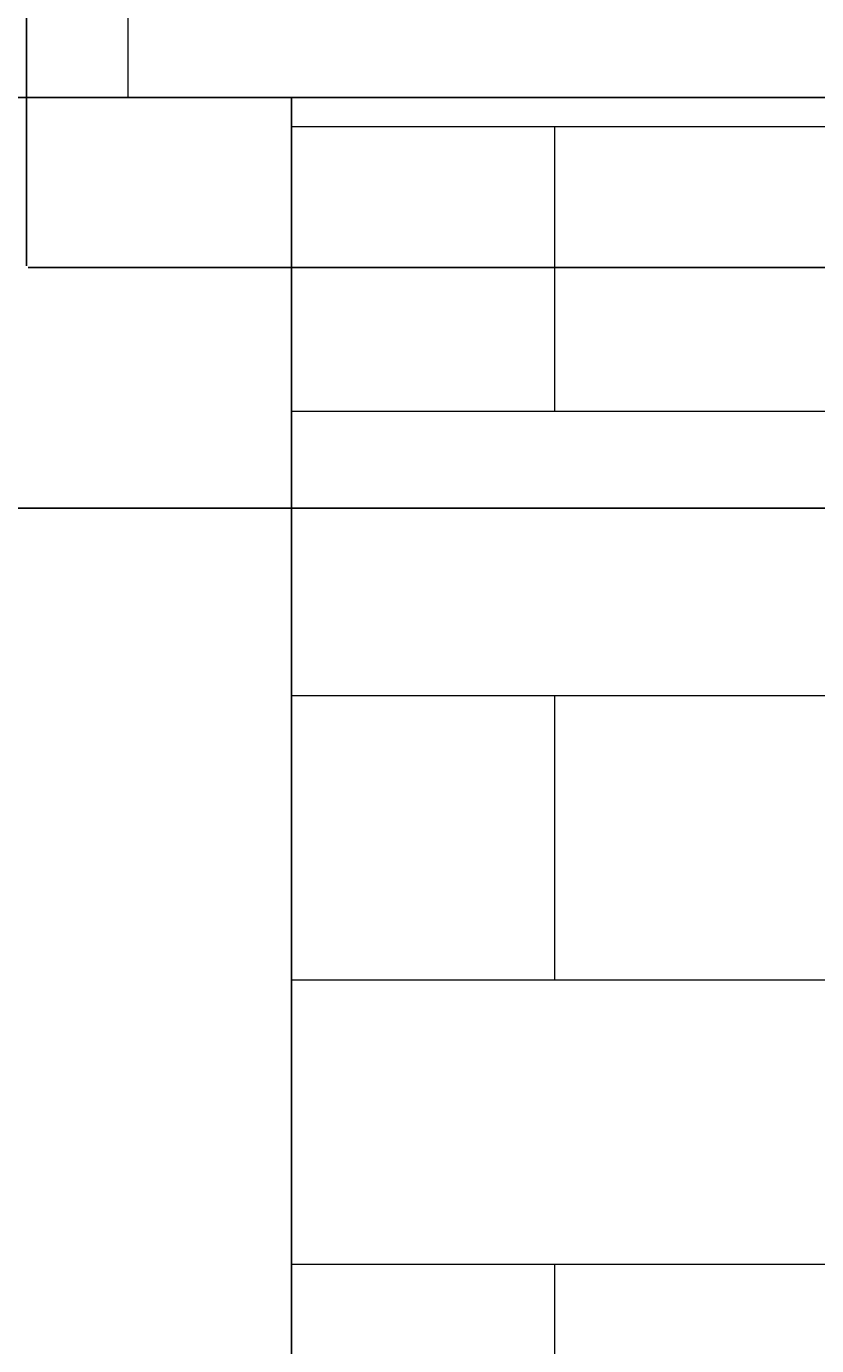
# Model space of a CAD drawing. Units: inches. Extents: x 37 to 824, y -700 to 234.
# Tile 18 of 77: x 348 to 378, y -536 to -487. Entities that reach past the tile are written whole.
import ezdxf

# ---------------------------------------------------------------- set-up
doc = ezdxf.new("R2010")
doc.units = ezdxf.units.IN
doc.header["$MEASUREMENT"] = 0
for name, color, linetype, lineweight in [('A-ANNO-DIMS', 2, 'Continuous', 18), ('A-ELEV', 3, 'Continuous', 25), ('A-ELEV-PATT', 8, 'Continuous', 13)]:
    doc.layers.add(name, color=color, linetype=linetype, lineweight=lineweight)
doc.styles.get("Standard").update_dxf_attribs({"font": 'arial.ttf'})
doc.dimstyles.get("Standard").update_dxf_attribs({"dimtxt": 0.18, "dimasz": 0.18, "dimexe": 0.18, "dimexo": 0.0625, "dimgap": 0.09, "dimtad": 0, "dimtih": 1, "dimtoh": 1, "dimdec": 1, "dimzin": 0, "dimdsep": 46, "dimlunit": 4, "dimtxsty": 'Standard', "dimcen": 0.09, "dimadec": 0, "dimazin": 0, "dimtfac": 1, "dimtdec": 1, "dimtofl": 0, "dimtmove": 0, "dimatfit": 3, "dimfxl": 1, "dimtolj": 1, "dimtzin": 0, "dimarcsym": 0})

# ---------------------------------------------------------------- blocks, each defined once
blk = doc.blocks.new('*D31')
at = {"layer": 'A-ANNO-DIMS', "color": 0, "lineweight": -2, "ltscale": 0.5, "transparency": 16777216}
for p, q in [((255.14, -489.627), (449.772, -489.627)), ((449.592, -495.627), (449.592, -510.537)), ((449.592, -531.627), (449.592, -516.717)), ((255.14, -537.627), (449.772, -537.627))]:
    blk.add_line(p, q, dxfattribs=at)
at = {"layer": 'A-ANNO-DIMS', "color": 0, "ltscale": 0.5, "transparency": 16777216}
for points in [[(448.592, -495.627), (450.592, -495.627), (449.592, -489.627)], [(448.592, -531.627), (450.592, -531.627), (449.592, -537.627)]]:
    blk.add_solid(points, dxfattribs=at)
at = {"layer": 'Defpoints', "color": 0, "ltscale": 0.5, "transparency": 16777216}
for p in [(255.077, -489.627), (449.592, -489.627), (255.077, -537.627)]:
    blk.add_point(p, dxfattribs=at)
at = {"layer": 'A-ANNO-DIMS', "color": 0, "ltscale": 0.5, "transparency": 16777216, "insert": (449.592, -513.627), "char_height": 6, "attachment_point": 5}
blk.add_mtext("\\A1;4'", dxfattribs=at)
blk = doc.blocks.new('*D99')
at = {"layer": 'A-ANNO-DIMS', "color": 0, "lineweight": -2, "ltscale": 0.5, "transparency": 16777216}
for p, q in [((308.196, -495.944), (308.196, -378.38)), ((348.196, -495.944), (348.196, -378.38)), ((308.376, -378.56), (327.866, -378.56)), ((348.016, -378.56), (328.525, -378.56))]:
    blk.add_line(p, q, dxfattribs=at)
at = {"layer": 'A-ANNO-DIMS', "color": 0, "ltscale": 0.5, "transparency": 16777216}
for points in [[(308.376, -378.53), (308.376, -378.59), (308.196, -378.56)], [(348.016, -378.53), (348.016, -378.59), (348.196, -378.56)]]:
    blk.add_solid(points, dxfattribs=at)
at = {"layer": 'Defpoints', "color": 0, "ltscale": 0.5, "transparency": 16777216}
for p in [(348.196, -378.56), (308.196, -496.007), (348.196, -496.007)]:
    blk.add_point(p, dxfattribs=at)
at = {"layer": 'A-ANNO-DIMS', "color": 0, "ltscale": 0.5, "transparency": 16777216, "insert": (328.196, -378.56), "char_height": 0.18, "attachment_point": 5}
blk.add_mtext('\\A1;3\'-4"', dxfattribs=at)
blk = doc.blocks.new('*D100')
at = {"layer": 'A-ANNO-DIMS', "color": 0, "lineweight": -2, "ltscale": 0.5, "transparency": 16777216}
for p, q in [((358.195, -489.627), (556.923, -489.627)), ((556.743, -489.807), (556.743, -492.634)), ((556.743, -495.827), (556.743, -493)), ((348.258, -496.007), (556.923, -496.007))]:
    blk.add_line(p, q, dxfattribs=at)
at = {"layer": 'A-ANNO-DIMS', "color": 0, "ltscale": 0.5, "transparency": 16777216}
for points in [[(556.713, -489.807), (556.773, -489.807), (556.743, -489.627)], [(556.713, -495.827), (556.773, -495.827), (556.743, -496.007)]]:
    blk.add_solid(points, dxfattribs=at)
at = {"layer": 'Defpoints', "color": 0, "ltscale": 0.5, "transparency": 16777216}
for p in [(358.132, -489.627), (348.196, -496.007), (556.743, -496.007)]:
    blk.add_point(p, dxfattribs=at)
at = {"layer": 'A-ANNO-DIMS', "color": 0, "ltscale": 0.5, "transparency": 16777216, "insert": (556.743, -492.817), "char_height": 0.18, "attachment_point": 5}
blk.add_mtext('\\A1;0\'-6 1/2"', dxfattribs=at)
blk = doc.blocks.new('*D101')
at = {"layer": 'A-ANNO-DIMS', "color": 0, "lineweight": -2, "ltscale": 0.5, "transparency": 16777216}
for p, q in [((348.258, -496.007), (556.923, -496.007)), ((556.743, -496.187), (556.743, -537.825)), ((556.743, -579.827), (556.743, -538.189)), ((348.258, -580.007), (556.923, -580.007))]:
    blk.add_line(p, q, dxfattribs=at)
at = {"layer": 'A-ANNO-DIMS', "color": 0, "ltscale": 0.5, "transparency": 16777216}
for points in [[(556.713, -496.187), (556.773, -496.187), (556.743, -496.007)], [(556.713, -579.827), (556.773, -579.827), (556.743, -580.007)]]:
    blk.add_solid(points, dxfattribs=at)
at = {"layer": 'Defpoints', "color": 0, "ltscale": 0.5, "transparency": 16777216}
for p in [(348.196, -496.007), (348.196, -580.007), (556.743, -580.007)]:
    blk.add_point(p, dxfattribs=at)
at = {"layer": 'A-ANNO-DIMS', "color": 0, "ltscale": 0.5, "transparency": 16777216, "insert": (556.743, -538.007), "char_height": 0.18, "attachment_point": 5}
blk.add_mtext('\\A1;7\'-0"', dxfattribs=at)
blk = doc.blocks.new('*D104')
at = {"layer": 'A-ANNO-DIMS', "color": 0, "lineweight": -2, "ltscale": 0.5, "transparency": 16777216}
for p, q in [((341.258, -505.03), (556.923, -505.03)), ((556.743, -505.21), (556.743, -539.336)), ((556.743, -573.827), (556.743, -539.7)), ((341.258, -574.007), (556.923, -574.007))]:
    blk.add_line(p, q, dxfattribs=at)
at = {"layer": 'A-ANNO-DIMS', "color": 0, "ltscale": 0.5, "transparency": 16777216}
for points in [[(556.713, -505.21), (556.773, -505.21), (556.743, -505.03)], [(556.713, -573.827), (556.773, -573.827), (556.743, -574.007)]]:
    blk.add_solid(points, dxfattribs=at)
at = {"layer": 'Defpoints', "color": 0, "ltscale": 0.5, "transparency": 16777216}
for p in [(341.196, -505.03), (341.196, -574.007), (556.743, -574.007)]:
    blk.add_point(p, dxfattribs=at)
at = {"layer": 'A-ANNO-DIMS', "color": 0, "ltscale": 0.5, "transparency": 16777216, "insert": (556.743, -539.518), "char_height": 0.18, "attachment_point": 5}
blk.add_mtext('\\A1;5\'-9"', dxfattribs=at)

msp = doc.modelspace()

# ---------------------------------------------------------------- hatches: boundary and pattern name
at = {"layer": 'A-ELEV-PATT', "ltscale": 0.5}
h = msp.add_hatch(dxfattribs=at)
h.set_pattern_fill('AR-BRSTD', color=256, scale=4)
h.paths.add_polyline_path([(299.077, -489.627), (358.132, -489.627), (358.132, -585.627), (428.077, -585.627), (428.077, -465.627), (161.077, -465.627), (161.077, -585.627), (299.077, -585.627)])
h.paths.add_polyline_path([(205.077, -537.627), (205.077, -489.627), (255.077, -489.627), (255.077, -537.627)], flags=16)

# ---------------------------------------------------------------- linework, layer by layer
at = {"layer": 'A-ELEV', "ltscale": 0.5}
msp.add_lwpolyline([(299.077, -489.627), (358.132, -489.627), (358.132, -585.627), (299.077, -585.627)], close=True, dxfattribs=at)

# ---------------------------------------------------------------- dimensions: what is measured, and where the dimension line sits
at = {"layer": 'A-ANNO-DIMS', "ltscale": 0.5}
dim = msp.add_linear_dim(base=(348.196, -378.56), p1=(308.196, -496.007), p2=(348.196, -496.007), dimstyle='Standard', override={"dimdec": 1, "dimlfac": 1, "dimrnd": 0, "dimzin": 1, "dimdsep": 46, "dimlunit": 4, "dimfrac": 2}, dxfattribs=at)
dim.commit()
dim.dimension.update_dxf_attribs({"geometry": '*D99', "text_midpoint": (328.196, -378.56)})
for base, p1, p2, override, picture, middle in [((449.592, -489.627), (255.077, -537.627), (255.077, -489.627), {"dimtxt": 6, "dimasz": 6, "dimclrd": 0, "dimclre": 0, "dimclrt": 0}, '*D31', (449.592, -513.627)), ((556.743, -496.007), (358.132, -489.627), (348.196, -496.007), {"dimdec": 1, "dimlfac": 1, "dimrnd": 0, "dimzin": 1, "dimdsep": 46, "dimlunit": 4, "dimfrac": 2}, '*D100', (556.743, -492.817)), ((556.743, -580.007), (348.196, -496.007), (348.196, -580.007), {"dimdec": 1, "dimlfac": 1, "dimrnd": 0, "dimzin": 1, "dimdsep": 46, "dimlunit": 4, "dimfrac": 2}, '*D101', (556.743, -538.007)), ((556.743, -574.007), (341.196, -505.03), (341.196, -574.007), {"dimdec": 1, "dimlfac": 1, "dimrnd": 0, "dimzin": 1, "dimdsep": 46, "dimlunit": 4, "dimfrac": 2}, '*D104', (556.743, -539.518))]:
    dim = msp.add_linear_dim(base=base, p1=p1, p2=p2, angle=90, dimstyle='Standard', override=override, dxfattribs=at)
    dim.commit()
    dim.dimension.update_dxf_attribs({"geometry": picture, "text_midpoint": middle})

doc.saveas('drawing.dxf')
